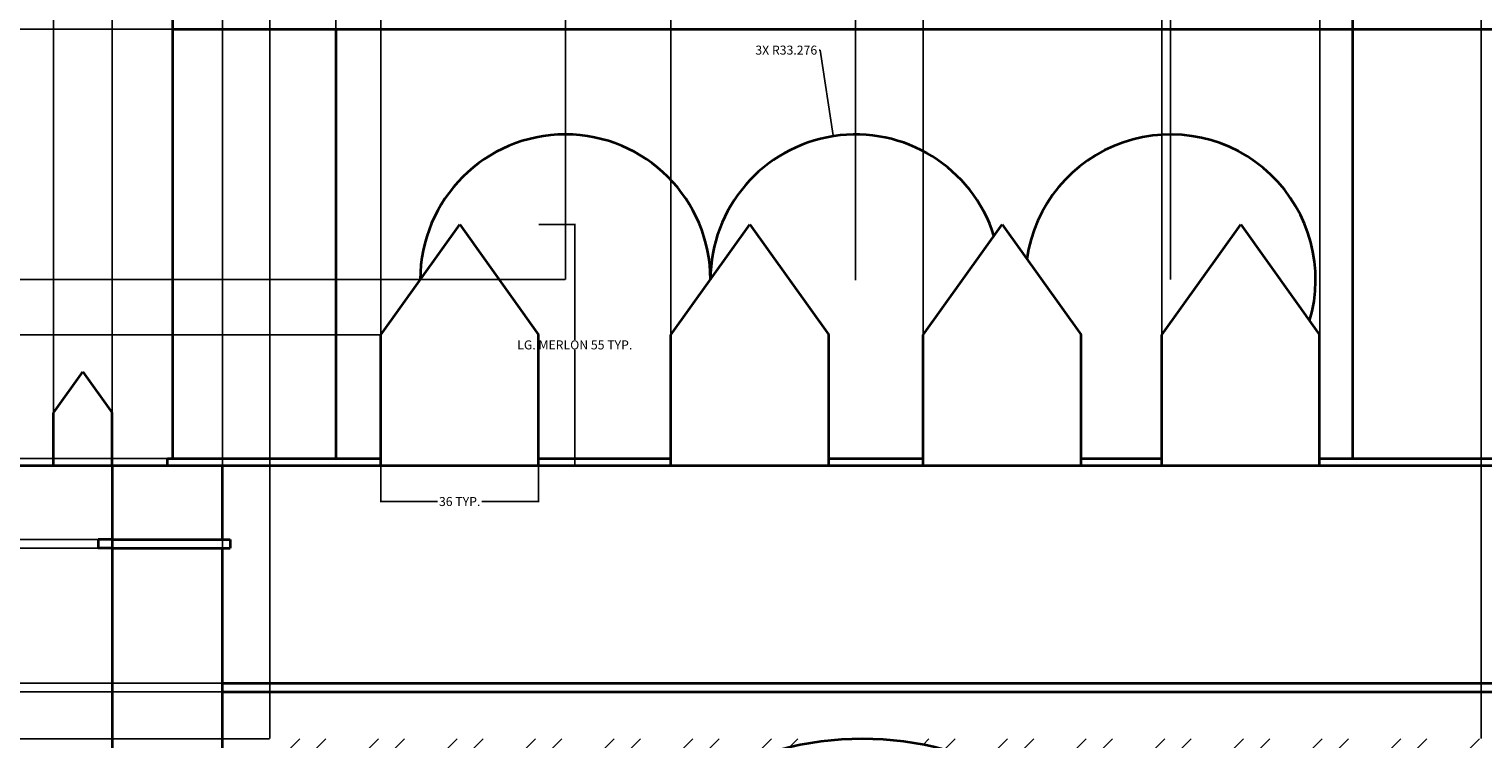
# Model space of a CAD drawing. Units: inches. Extents: x 14 to 859, y 52 to 711.
# Tile 5 of 11: x 244 to 577, y 342 to 504. Entities that reach past the tile are written whole.
import ezdxf

# ---------------------------------------------------------------- set-up
doc = ezdxf.new("R2010")
doc.units = ezdxf.units.IN
doc.header["$MEASUREMENT"] = 0
for name, color, linetype, lineweight in [('A-ANNO-DIMS', 2, 'Continuous', 18), ('A-ELEV', 7, 'Continuous', 35), ('A-ELEV-PATT', 8, 'Continuous', 13)]:
    doc.layers.add(name, color=color, linetype=linetype, lineweight=lineweight)
doc.styles.get("Standard").update_dxf_attribs({"font": 'arial.ttf'})
doc.dimstyles.get("Standard").update_dxf_attribs({"dimtxt": 2.0625, "dimasz": 0.18, "dimexe": 0.18, "dimexo": 0.0625, "dimgap": 0.09, "dimtad": 0, "dimtih": 1, "dimtoh": 1, "dimdec": 4, "dimzin": 0, "dimdsep": 46, "dimlunit": 4, "dimtxsty": 'Standard', "dimcen": 0.09, "dimadec": 0, "dimazin": 0, "dimtfac": 1, "dimtdec": 4, "dimtofl": 0, "dimtmove": 0, "dimatfit": 3, "dimfxl": 1, "dimtolj": 1, "dimtzin": 0, "dimarcsym": 0})

# ---------------------------------------------------------------- blocks, each defined once
blk = doc.blocks.new('MERLON-LARGE')
for p, q in [((0, 29.92), (18.11, 55.24)), ((18.11, 55.24), (36.21, 29.92)), ((0, 0), (0, 29.92)), ((36.21, 0), (36.21, 29.92))]:
    blk.add_line(p, q)
blk = doc.blocks.new('*D9')
at = {"layer": 'A-ANNO-DIMS', "color": 0, "lineweight": -2, "transparency": 16777216}
for p, q in [((360.45, 459.61), (368.85, 459.61)), ((368.67, 459.43), (368.67, 433.15)), ((368.67, 404.55), (368.67, 430.83)), ((360.45, 404.37), (368.85, 404.37))]:
    blk.add_line(p, q, dxfattribs=at)
at = {"layer": 'A-ANNO-DIMS', "color": 0, "transparency": 16777216}
for points in [[(368.64, 459.43), (368.7, 459.43), (368.67, 459.61)], [(368.64, 404.55), (368.7, 404.55), (368.67, 404.37)]]:
    blk.add_solid(points, dxfattribs=at)
at = {"layer": 'Defpoints', "color": 0, "transparency": 16777216}
for p in [(360.39, 459.61), (368.67, 459.61), (360.39, 404.37)]:
    blk.add_point(p, dxfattribs=at)
at = {"layer": 'A-ANNO-DIMS', "color": 0, "transparency": 16777216, "insert": (368.67, 431.99), "char_height": 2.0625, "attachment_point": 5}
blk.add_mtext('\\A1;LG. MERLON 55 TYP.', dxfattribs=at)
blk = doc.blocks.new('*D10')
at = {"layer": 'A-ANNO-DIMS', "color": 0, "lineweight": -2, "transparency": 16777216}
for p, q in [((324.18, 404.31), (324.18, 395.91)), ((360.39, 404.31), (360.39, 395.91)), ((324.36, 396.09), (337.17, 396.09)), ((360.21, 396.09), (347.39, 396.09))]:
    blk.add_line(p, q, dxfattribs=at)
at = {"layer": 'A-ANNO-DIMS', "color": 0, "transparency": 16777216}
for points in [[(324.36, 396.12), (324.36, 396.06), (324.18, 396.09)], [(360.21, 396.12), (360.21, 396.06), (360.39, 396.09)]]:
    blk.add_solid(points, dxfattribs=at)
at = {"layer": 'Defpoints', "color": 0, "transparency": 16777216}
for p in [(324.18, 404.37), (360.39, 404.37), (360.39, 396.09)]:
    blk.add_point(p, dxfattribs=at)
at = {"layer": 'A-ANNO-DIMS', "color": 0, "transparency": 16777216, "insert": (342.28, 396.09), "char_height": 2.0625, "attachment_point": 5}
blk.add_mtext('\\A1;36 TYP.', dxfattribs=at)
blk = doc.blocks.new('*D13')
at = {"layer": 'A-ANNO-DIMS', "color": 0, "lineweight": -2, "transparency": 16777216}
for p, q in [((60.78, 339.73), (60.78, 709.71)), ((60.96, 709.53), (432.6, 709.53)), ((811.37, 709.53), (439.73, 709.53)), ((811.55, 339.73), (811.55, 709.71))]:
    blk.add_line(p, q, dxfattribs=at)
at = {"layer": 'A-ANNO-DIMS', "color": 0, "transparency": 16777216}
for points in [[(60.96, 709.56), (60.96, 709.5), (60.78, 709.53)], [(811.37, 709.56), (811.37, 709.5), (811.55, 709.53)]]:
    blk.add_solid(points, dxfattribs=at)
at = {"layer": 'Defpoints', "color": 0, "transparency": 16777216}
for p in [(811.55, 709.53), (60.78, 339.66), (811.55, 339.66)]:
    blk.add_point(p, dxfattribs=at)
at = {"layer": 'A-ANNO-DIMS', "color": 0, "transparency": 16777216, "insert": (436.17, 709.53), "char_height": 2.062, "attachment_point": 5}
blk.add_mtext('\\A1;750.8', dxfattribs=at)
blk = doc.blocks.new('*D16')
at = {"layer": 'A-ANNO-DIMS', "color": 0, "lineweight": -2, "transparency": 16777216}
for p, q in [((429.96, 670.76), (17.7, 670.76)), ((17.88, 670.58), (17.88, 384.41)), ((17.88, 95.97), (17.88, 382.14)), ((60.72, 95.79), (17.7, 95.79))]:
    blk.add_line(p, q, dxfattribs=at)
at = {"layer": 'A-ANNO-DIMS', "color": 0, "transparency": 16777216}
for points in [[(17.85, 670.58), (17.91, 670.58), (17.88, 670.76)], [(17.85, 95.97), (17.91, 95.97), (17.88, 95.79)]]:
    blk.add_solid(points, dxfattribs=at)
at = {"layer": 'Defpoints', "color": 0, "transparency": 16777216}
for p in [(17.88, 670.76), (430.02, 670.76), (60.78, 95.79)]:
    blk.add_point(p, dxfattribs=at)
at = {"layer": 'A-ANNO-DIMS', "color": 0, "transparency": 16777216, "insert": (17.88, 383.28), "char_height": 2.062, "attachment_point": 5}
blk.add_mtext('\\A1;575', dxfattribs=at)
blk = doc.blocks.new('*D19')
at = {"layer": 'A-ANNO-DIMS', "color": 0, "lineweight": -2, "transparency": 16777216}
for p, q in [((430.09, 670.76), (854.64, 670.76)), ((854.46, 670.58), (854.46, 538.71)), ((854.46, 404.55), (854.46, 536.42)), ((609.81, 404.37), (854.64, 404.37))]:
    blk.add_line(p, q, dxfattribs=at)
at = {"layer": 'A-ANNO-DIMS', "color": 0, "transparency": 16777216}
for points in [[(854.43, 670.58), (854.49, 670.58), (854.46, 670.76)], [(854.43, 404.55), (854.49, 404.55), (854.46, 404.37)]]:
    blk.add_solid(points, dxfattribs=at)
at = {"layer": 'Defpoints', "color": 0, "transparency": 16777216}
for p in [(430.02, 670.76), (854.46, 670.76), (609.75, 404.37)]:
    blk.add_point(p, dxfattribs=at)
at = {"layer": 'A-ANNO-DIMS', "color": 0, "transparency": 16777216, "insert": (854.46, 537.57), "char_height": 2.062, "attachment_point": 5}
blk.add_mtext('\\A1;266.4', dxfattribs=at)
blk = doc.blocks.new('*D21')
at = {"layer": 'A-ANNO-DIMS', "color": 0, "lineweight": -2, "transparency": 16777216}
for p, q in [((287.89, 352.49), (287.89, 709.71)), ((288.07, 709.53), (289.04, 709.53)), ((298.55, 709.53), (297.59, 709.53)), ((298.73, 341.73), (298.73, 709.71))]:
    blk.add_line(p, q, dxfattribs=at)
at = {"layer": 'A-ANNO-DIMS', "color": 0, "transparency": 16777216}
for points in [[(288.07, 709.56), (288.07, 709.5), (287.89, 709.53)], [(298.55, 709.56), (298.55, 709.5), (298.73, 709.53)]]:
    blk.add_solid(points, dxfattribs=at)
at = {"layer": 'Defpoints', "color": 0, "transparency": 16777216}
for p in [(298.73, 709.53), (287.89, 352.43), (298.73, 341.67)]:
    blk.add_point(p, dxfattribs=at)
at = {"layer": 'A-ANNO-DIMS', "color": 0, "transparency": 16777216, "insert": (293.31, 709.53), "char_height": 2.062, "attachment_point": 5}
blk.add_mtext('\\A1;10.837', dxfattribs=at)
blk = doc.blocks.new('*D22')
at = {"layer": 'A-ANNO-DIMS', "color": 0, "lineweight": -2, "transparency": 16777216}
for p, q in [((298.73, 341.73), (298.73, 709.71)), ((298.91, 709.53), (434.03, 709.53)), ((576.33, 709.53), (441.21, 709.53)), ((576.51, 341.73), (576.51, 709.71))]:
    blk.add_line(p, q, dxfattribs=at)
at = {"layer": 'A-ANNO-DIMS', "color": 0, "transparency": 16777216}
for points in [[(298.91, 709.56), (298.91, 709.5), (298.73, 709.53)], [(576.33, 709.56), (576.33, 709.5), (576.51, 709.53)]]:
    blk.add_solid(points, dxfattribs=at)
at = {"layer": 'Defpoints', "color": 0, "transparency": 16777216}
for p in [(576.51, 709.53), (298.73, 341.67), (576.51, 341.67)]:
    blk.add_point(p, dxfattribs=at)
at = {"layer": 'A-ANNO-DIMS', "color": 0, "transparency": 16777216, "insert": (437.62, 709.53), "char_height": 2.062, "attachment_point": 5}
blk.add_mtext('\\A1;277.8', dxfattribs=at)
blk = doc.blocks.new('*D23')
at = {"layer": 'A-ANNO-DIMS', "color": 0, "lineweight": -2, "transparency": 16777216}
for p, q in [((576.51, 341.73), (576.51, 709.71)), ((576.69, 709.53), (576.9, 709.53)), ((584.26, 709.53), (584.04, 709.53)), ((584.44, 352.49), (584.44, 709.71))]:
    blk.add_line(p, q, dxfattribs=at)
at = {"layer": 'A-ANNO-DIMS', "color": 0, "transparency": 16777216}
for points in [[(576.69, 709.56), (576.69, 709.5), (576.51, 709.53)], [(584.26, 709.56), (584.26, 709.5), (584.44, 709.53)]]:
    blk.add_solid(points, dxfattribs=at)
at = {"layer": 'Defpoints', "color": 0, "transparency": 16777216}
for p in [(584.44, 709.53), (584.44, 352.43), (576.51, 341.67)]:
    blk.add_point(p, dxfattribs=at)
at = {"layer": 'A-ANNO-DIMS', "color": 0, "transparency": 16777216, "insert": (580.47, 709.53), "char_height": 2.062, "attachment_point": 5}
blk.add_mtext('\\A1;7.935', dxfattribs=at)
blk = doc.blocks.new('*D25')
at = {"layer": 'A-ANNO-DIMS', "color": 0, "lineweight": -2, "transparency": 16777216}
for p, q in [((298.67, 341.67), (17.7, 341.67)), ((17.88, 341.49), (17.88, 305.98)), ((17.88, 268.19), (17.88, 303.7)), ((298.67, 268.01), (17.7, 268.01))]:
    blk.add_line(p, q, dxfattribs=at)
at = {"layer": 'A-ANNO-DIMS', "color": 0, "transparency": 16777216}
for points in [[(17.85, 341.49), (17.91, 341.49), (17.88, 341.67)], [(17.85, 268.19), (17.91, 268.19), (17.88, 268.01)]]:
    blk.add_solid(points, dxfattribs=at)
at = {"layer": 'Defpoints', "color": 0, "transparency": 16777216}
for p in [(17.88, 341.67), (298.73, 341.67), (298.73, 268.01)]:
    blk.add_point(p, dxfattribs=at)
at = {"layer": 'A-ANNO-DIMS', "color": 0, "transparency": 16777216, "insert": (17.88, 304.84), "char_height": 2.062, "attachment_point": 5}
blk.add_mtext('\\A1;73.66', dxfattribs=at)
blk = doc.blocks.new('*D26')
at = {"layer": 'A-ANNO-DIMS', "color": 0, "lineweight": -2, "transparency": 16777216}
for p, q in [((287.83, 352.43), (17.7, 352.43)), ((17.88, 352.25), (17.88, 348.19)), ((17.88, 341.85), (17.88, 345.91)), ((298.67, 341.67), (17.7, 341.67))]:
    blk.add_line(p, q, dxfattribs=at)
at = {"layer": 'A-ANNO-DIMS', "color": 0, "transparency": 16777216}
for points in [[(17.85, 352.25), (17.91, 352.25), (17.88, 352.43)], [(17.85, 341.85), (17.91, 341.85), (17.88, 341.67)]]:
    blk.add_solid(points, dxfattribs=at)
at = {"layer": 'Defpoints', "color": 0, "transparency": 16777216}
for p in [(17.88, 352.43), (287.89, 352.43), (298.73, 341.67)]:
    blk.add_point(p, dxfattribs=at)
at = {"layer": 'A-ANNO-DIMS', "color": 0, "transparency": 16777216, "insert": (17.88, 347.05), "char_height": 2.062, "attachment_point": 5}
blk.add_mtext('\\A1;10.758', dxfattribs=at)
blk = doc.blocks.new('*D27')
at = {"layer": 'A-ANNO-DIMS', "color": 0, "lineweight": -2, "transparency": 16777216}
for p, q in [((287.83, 354.43), (17.7, 354.43)), ((17.88, 354.43), (17.88, 354.61)), ((17.88, 354.61), (18.06, 354.61)), ((17.88, 352.61), (17.88, 354.25)), ((287.83, 352.43), (17.7, 352.43))]:
    blk.add_line(p, q, dxfattribs=at)
at = {"layer": 'A-ANNO-DIMS', "color": 0, "transparency": 16777216}
for points in [[(17.85, 354.25), (17.91, 354.25), (17.88, 354.43)], [(17.85, 352.61), (17.91, 352.61), (17.88, 352.43)]]:
    blk.add_solid(points, dxfattribs=at)
at = {"layer": 'Defpoints', "color": 0, "transparency": 16777216}
for p in [(17.88, 354.43), (287.89, 354.43), (287.89, 352.43)]:
    blk.add_point(p, dxfattribs=at)
at = {"layer": 'A-ANNO-DIMS', "color": 0, "transparency": 16777216, "insert": (18.83, 354.61), "char_height": 2.062, "attachment_point": 5}
blk.add_mtext('\\A1;2', dxfattribs=at)
blk = doc.blocks.new('*D28')
at = {"layer": 'A-ANNO-DIMS', "color": 0, "lineweight": -2, "transparency": 16777216}
for p, q in [((289.61, 385.4), (17.7, 385.4)), ((17.88, 385.22), (17.88, 371.06)), ((17.88, 354.61), (17.88, 368.77)), ((287.83, 354.43), (17.7, 354.43))]:
    blk.add_line(p, q, dxfattribs=at)
at = {"layer": 'A-ANNO-DIMS', "color": 0, "transparency": 16777216}
for points in [[(17.85, 385.22), (17.91, 385.22), (17.88, 385.4)], [(17.85, 354.61), (17.91, 354.61), (17.88, 354.43)]]:
    blk.add_solid(points, dxfattribs=at)
at = {"layer": 'Defpoints', "color": 0, "transparency": 16777216}
for p in [(17.88, 385.4), (289.67, 385.4), (287.89, 354.43)]:
    blk.add_point(p, dxfattribs=at)
at = {"layer": 'A-ANNO-DIMS', "color": 0, "transparency": 16777216, "insert": (17.88, 369.91), "char_height": 2.062, "attachment_point": 5}
blk.add_mtext('\\A1;30.97', dxfattribs=at)
blk = doc.blocks.new('*D29')
at = {"layer": 'A-ANNO-DIMS', "color": 0, "lineweight": -2, "transparency": 16777216}
for p, q in [((289.61, 387.4), (17.7, 387.4)), ((17.88, 387.4), (17.88, 387.58)), ((17.88, 387.58), (18.06, 387.58)), ((17.88, 385.58), (17.88, 387.22)), ((289.61, 385.4), (17.7, 385.4))]:
    blk.add_line(p, q, dxfattribs=at)
at = {"layer": 'A-ANNO-DIMS', "color": 0, "transparency": 16777216}
for points in [[(17.85, 387.22), (17.91, 387.22), (17.88, 387.4)], [(17.85, 385.58), (17.91, 385.58), (17.88, 385.4)]]:
    blk.add_solid(points, dxfattribs=at)
at = {"layer": 'Defpoints', "color": 0, "transparency": 16777216}
for p in [(17.88, 387.4), (289.67, 387.4), (289.67, 385.4)]:
    blk.add_point(p, dxfattribs=at)
at = {"layer": 'A-ANNO-DIMS', "color": 0, "transparency": 16777216, "insert": (18.83, 387.58), "char_height": 2.062, "attachment_point": 5}
blk.add_mtext('\\A1;2', dxfattribs=at)
blk = doc.blocks.new('*D30')
at = {"layer": 'A-ANNO-DIMS', "color": 0, "lineweight": -2, "transparency": 16777216}
for p, q in [((287.83, 404.37), (17.7, 404.37)), ((17.88, 404.19), (17.88, 397.03)), ((17.88, 387.58), (17.88, 394.74)), ((289.61, 387.4), (17.7, 387.4))]:
    blk.add_line(p, q, dxfattribs=at)
at = {"layer": 'A-ANNO-DIMS', "color": 0, "transparency": 16777216}
for points in [[(17.85, 404.19), (17.91, 404.19), (17.88, 404.37)], [(17.85, 387.58), (17.91, 387.58), (17.88, 387.4)]]:
    blk.add_solid(points, dxfattribs=at)
at = {"layer": 'Defpoints', "color": 0, "transparency": 16777216}
for p in [(17.88, 404.37), (287.89, 404.37), (289.67, 387.4)]:
    blk.add_point(p, dxfattribs=at)
at = {"layer": 'A-ANNO-DIMS', "color": 0, "transparency": 16777216, "insert": (17.88, 395.88), "char_height": 2.062, "attachment_point": 5}
blk.add_mtext('\\A1;16.973', dxfattribs=at)
blk = doc.blocks.new('*D66')
at = {"layer": 'A-ANNO-DIMS', "color": 0, "lineweight": -2, "transparency": 16777216}
for p, q in [((223.53, 404.43), (223.53, 709.71)), ((223.71, 709.53), (232.77, 709.53)), ((249.01, 709.53), (239.95, 709.53)), ((249.19, 404.43), (249.19, 709.71))]:
    blk.add_line(p, q, dxfattribs=at)
at = {"layer": 'A-ANNO-DIMS', "color": 0, "transparency": 16777216}
for points in [[(223.71, 709.56), (223.71, 709.5), (223.53, 709.53)], [(249.01, 709.56), (249.01, 709.5), (249.19, 709.53)]]:
    blk.add_solid(points, dxfattribs=at)
at = {"layer": 'Defpoints', "color": 0, "transparency": 16777216}
for p in [(249.19, 709.53), (223.53, 404.37), (249.19, 404.37)]:
    blk.add_point(p, dxfattribs=at)
at = {"layer": 'A-ANNO-DIMS', "color": 0, "transparency": 16777216, "insert": (236.36, 709.53), "char_height": 2.062, "attachment_point": 5}
blk.add_mtext('\\A1;25.67', dxfattribs=at)
blk = doc.blocks.new('*D67')
at = {"layer": 'A-ANNO-DIMS', "color": 0, "lineweight": -2, "transparency": 16777216}
for p, q in [((249.19, 404.43), (249.19, 709.71)), ((249.37, 709.53), (252.41, 709.53)), ((262.4, 709.53), (259.36, 709.53)), ((262.58, 404.43), (262.58, 709.71))]:
    blk.add_line(p, q, dxfattribs=at)
at = {"layer": 'A-ANNO-DIMS', "color": 0, "transparency": 16777216}
for points in [[(249.37, 709.56), (249.37, 709.5), (249.19, 709.53)], [(262.4, 709.56), (262.4, 709.5), (262.58, 709.53)]]:
    blk.add_solid(points, dxfattribs=at)
at = {"layer": 'Defpoints', "color": 0, "transparency": 16777216}
for p in [(262.58, 709.53), (249.19, 404.37), (262.58, 404.37)]:
    blk.add_point(p, dxfattribs=at)
at = {"layer": 'A-ANNO-DIMS', "color": 0, "transparency": 16777216, "insert": (255.89, 709.53), "char_height": 2.062, "attachment_point": 5}
blk.add_mtext('\\A1;13.39', dxfattribs=at)
blk = doc.blocks.new('*D86')
at = {"layer": 'A-ANNO-DIMS', "color": 0, "lineweight": -2, "transparency": 16777216}
for p, q in [((366.44, 446.95), (17.7, 446.95)), ((17.88, 446.77), (17.88, 427.59)), ((17.88, 406.12), (17.88, 425.3)), ((276.44, 405.94), (17.7, 405.94))]:
    blk.add_line(p, q, dxfattribs=at)
at = {"layer": 'A-ANNO-DIMS', "color": 0, "transparency": 16777216}
for points in [[(17.85, 446.77), (17.91, 446.77), (17.88, 446.95)], [(17.85, 406.12), (17.91, 406.12), (17.88, 405.94)]]:
    blk.add_solid(points, dxfattribs=at)
at = {"layer": 'Defpoints', "color": 0, "transparency": 16777216}
for p in [(17.88, 446.95), (366.51, 446.95), (276.5, 405.94)]:
    blk.add_point(p, dxfattribs=at)
at = {"layer": 'A-ANNO-DIMS', "color": 0, "transparency": 16777216, "insert": (17.88, 426.45), "char_height": 2.062, "attachment_point": 5}
blk.add_mtext('\\A1;41.01', dxfattribs=at)
blk = doc.blocks.new('*D87')
at = {"layer": 'A-ANNO-DIMS', "color": 0, "lineweight": -2, "transparency": 16777216}
for p, q in [((276.44, 504.38), (17.7, 504.38)), ((17.88, 504.2), (17.88, 476.81)), ((17.88, 447.13), (17.88, 474.52)), ((366.44, 446.95), (17.7, 446.95))]:
    blk.add_line(p, q, dxfattribs=at)
at = {"layer": 'A-ANNO-DIMS', "color": 0, "transparency": 16777216}
for points in [[(17.85, 504.2), (17.91, 504.2), (17.88, 504.38)], [(17.85, 447.13), (17.91, 447.13), (17.88, 446.95)]]:
    blk.add_solid(points, dxfattribs=at)
at = {"layer": 'Defpoints', "color": 0, "transparency": 16777216}
for p in [(17.88, 504.38), (276.5, 504.38), (366.51, 446.95)]:
    blk.add_point(p, dxfattribs=at)
at = {"layer": 'A-ANNO-DIMS', "color": 0, "transparency": 16777216, "insert": (17.88, 475.67), "char_height": 2.062, "attachment_point": 5}
blk.add_mtext('\\A1;57.43', dxfattribs=at)
blk = doc.blocks.new('*D96')
at = {"layer": 'A-ANNO-DIMS', "color": 0, "lineweight": -2, "transparency": 16777216}
for p, q in [((313.86, 504.44), (313.86, 709.71)), ((314.04, 709.53), (336.61, 709.53)), ((366.33, 709.53), (343.76, 709.53)), ((366.51, 447.01), (366.51, 709.71))]:
    blk.add_line(p, q, dxfattribs=at)
at = {"layer": 'A-ANNO-DIMS', "color": 0, "transparency": 16777216}
for points in [[(314.04, 709.56), (314.04, 709.5), (313.86, 709.53)], [(366.33, 709.56), (366.33, 709.5), (366.51, 709.53)]]:
    blk.add_solid(points, dxfattribs=at)
at = {"layer": 'Defpoints', "color": 0, "transparency": 16777216}
for p in [(366.51, 709.53), (313.86, 504.38), (366.51, 446.95)]:
    blk.add_point(p, dxfattribs=at)
at = {"layer": 'A-ANNO-DIMS', "color": 0, "transparency": 16777216, "insert": (340.18, 709.53), "char_height": 2.062, "attachment_point": 5}
blk.add_mtext('\\A1;52.65', dxfattribs=at)
blk = doc.blocks.new('*D97')
at = {"layer": 'A-ANNO-DIMS', "color": 0, "lineweight": -2, "transparency": 16777216}
for p, q in [((366.51, 447.01), (366.51, 709.71)), ((366.69, 709.53), (396.2, 709.53)), ((432.88, 709.53), (403.37, 709.53)), ((433.06, 447.01), (433.06, 709.71))]:
    blk.add_line(p, q, dxfattribs=at)
at = {"layer": 'A-ANNO-DIMS', "color": 0, "transparency": 16777216}
for points in [[(366.69, 709.56), (366.69, 709.5), (366.51, 709.53)], [(432.88, 709.56), (432.88, 709.5), (433.06, 709.53)]]:
    blk.add_solid(points, dxfattribs=at)
at = {"layer": 'Defpoints', "color": 0, "transparency": 16777216}
for p in [(433.06, 709.53), (366.51, 446.95), (433.06, 446.95)]:
    blk.add_point(p, dxfattribs=at)
at = {"layer": 'A-ANNO-DIMS', "color": 0, "transparency": 16777216, "insert": (399.78, 709.53), "char_height": 2.062, "attachment_point": 5}
blk.add_mtext('\\A1;66.55', dxfattribs=at)
blk = doc.blocks.new('*D98')
at = {"layer": 'A-ANNO-DIMS', "color": 0, "lineweight": -2, "transparency": 16777216}
for p, q in [((433.06, 447.01), (433.06, 709.71)), ((433.24, 709.53), (465.59, 709.53)), ((505.07, 709.53), (472.72, 709.53)), ((505.25, 447.01), (505.25, 709.71))]:
    blk.add_line(p, q, dxfattribs=at)
at = {"layer": 'A-ANNO-DIMS', "color": 0, "transparency": 16777216}
for points in [[(433.24, 709.56), (433.24, 709.5), (433.06, 709.53)], [(505.07, 709.56), (505.07, 709.5), (505.25, 709.53)]]:
    blk.add_solid(points, dxfattribs=at)
at = {"layer": 'Defpoints', "color": 0, "transparency": 16777216}
for p in [(505.25, 709.53), (433.06, 446.95), (505.25, 446.95)]:
    blk.add_point(p, dxfattribs=at)
at = {"layer": 'A-ANNO-DIMS', "color": 0, "transparency": 16777216, "insert": (469.15, 709.53), "char_height": 2.062, "attachment_point": 5}
blk.add_mtext('\\A1;72.19', dxfattribs=at)
blk = doc.blocks.new('*D99')
at = {"layer": 'A-ANNO-DIMS', "color": 0, "lineweight": -2, "transparency": 16777216}
for p, q in [((505.25, 447.01), (505.25, 709.71)), ((505.43, 709.53), (521.76, 709.53)), ((546.91, 709.53), (530.58, 709.53)), ((547.09, 509.85), (547.09, 709.71))]:
    blk.add_line(p, q, dxfattribs=at)
at = {"layer": 'A-ANNO-DIMS', "color": 0, "transparency": 16777216}
for points in [[(505.43, 709.56), (505.43, 709.5), (505.25, 709.53)], [(546.91, 709.56), (546.91, 709.5), (547.09, 709.53)]]:
    blk.add_solid(points, dxfattribs=at)
at = {"layer": 'Defpoints', "color": 0, "transparency": 16777216}
for p in [(547.09, 709.53), (547.09, 509.79), (505.25, 446.95)]:
    blk.add_point(p, dxfattribs=at)
at = {"layer": 'A-ANNO-DIMS', "color": 0, "transparency": 16777216, "insert": (526.17, 709.53), "char_height": 2.062, "attachment_point": 5}
blk.add_mtext('\\A1;41.836', dxfattribs=at)
blk = doc.blocks.new('*D119')
at = {"layer": 'A-ANNO-DIMS', "color": 0, "lineweight": -2, "transparency": 16777216}
for p, q in [((287.89, 404.43), (287.89, 709.71)), ((288.07, 709.53), (301.66, 709.53)), ((324, 709.53), (310.41, 709.53)), ((324.18, 404.43), (324.18, 709.71))]:
    blk.add_line(p, q, dxfattribs=at)
at = {"layer": 'A-ANNO-DIMS', "color": 0, "transparency": 16777216}
for points in [[(288.07, 709.56), (288.07, 709.5), (287.89, 709.53)], [(324, 709.56), (324, 709.5), (324.18, 709.53)]]:
    blk.add_solid(points, dxfattribs=at)
at = {"layer": 'Defpoints', "color": 0, "transparency": 16777216}
for p in [(324.18, 709.53), (287.89, 404.37), (324.18, 404.37)]:
    blk.add_point(p, dxfattribs=at)
at = {"layer": 'A-ANNO-DIMS', "color": 0, "transparency": 16777216, "insert": (306.04, 709.53), "char_height": 2.062, "attachment_point": 5}
blk.add_mtext('\\A1;36.285', dxfattribs=at)
blk = doc.blocks.new('*D120')
at = {"layer": 'A-ANNO-DIMS', "color": 0, "lineweight": -2, "transparency": 16777216}
for p, q in [((324.18, 404.43), (324.18, 709.71)), ((324.36, 709.53), (353.87, 709.53)), ((390.55, 709.53), (361.04, 709.53)), ((390.73, 404.43), (390.73, 709.71))]:
    blk.add_line(p, q, dxfattribs=at)
at = {"layer": 'A-ANNO-DIMS', "color": 0, "transparency": 16777216}
for points in [[(324.36, 709.56), (324.36, 709.5), (324.18, 709.53)], [(390.55, 709.56), (390.55, 709.5), (390.73, 709.53)]]:
    blk.add_solid(points, dxfattribs=at)
at = {"layer": 'Defpoints', "color": 0, "transparency": 16777216}
for p in [(390.73, 709.53), (324.18, 404.37), (390.73, 404.37)]:
    blk.add_point(p, dxfattribs=at)
at = {"layer": 'A-ANNO-DIMS', "color": 0, "transparency": 16777216, "insert": (357.45, 709.53), "char_height": 2.062, "attachment_point": 5}
blk.add_mtext('\\A1;66.55', dxfattribs=at)
blk = doc.blocks.new('*D121')
at = {"layer": 'A-ANNO-DIMS', "color": 0, "lineweight": -2, "transparency": 16777216}
for p, q in [((390.73, 404.43), (390.73, 709.71)), ((390.91, 709.53), (416.86, 709.53)), ((448.36, 709.53), (422.4, 709.53)), ((448.54, 404.43), (448.54, 709.71))]:
    blk.add_line(p, q, dxfattribs=at)
at = {"layer": 'A-ANNO-DIMS', "color": 0, "transparency": 16777216}
for points in [[(390.91, 709.56), (390.91, 709.5), (390.73, 709.53)], [(448.36, 709.56), (448.36, 709.5), (448.54, 709.53)]]:
    blk.add_solid(points, dxfattribs=at)
at = {"layer": 'Defpoints', "color": 0, "transparency": 16777216}
for p in [(448.54, 709.53), (390.73, 404.37), (448.54, 404.37)]:
    blk.add_point(p, dxfattribs=at)
at = {"layer": 'A-ANNO-DIMS', "color": 0, "transparency": 16777216, "insert": (419.63, 709.53), "char_height": 2.062, "attachment_point": 5}
blk.add_mtext('\\A1;57.8', dxfattribs=at)
blk = doc.blocks.new('*D122')
at = {"layer": 'A-ANNO-DIMS', "color": 0, "lineweight": -2, "transparency": 16777216}
for p, q in [((448.54, 404.43), (448.54, 709.71)), ((448.72, 709.53), (473.12, 709.53)), ((503.05, 709.53), (478.65, 709.53)), ((503.23, 404.43), (503.23, 709.71))]:
    blk.add_line(p, q, dxfattribs=at)
at = {"layer": 'A-ANNO-DIMS', "color": 0, "transparency": 16777216}
for points in [[(448.72, 709.56), (448.72, 709.5), (448.54, 709.53)], [(503.05, 709.56), (503.05, 709.5), (503.23, 709.53)]]:
    blk.add_solid(points, dxfattribs=at)
at = {"layer": 'Defpoints', "color": 0, "transparency": 16777216}
for p in [(503.23, 709.53), (448.54, 404.37), (503.23, 404.37)]:
    blk.add_point(p, dxfattribs=at)
at = {"layer": 'A-ANNO-DIMS', "color": 0, "transparency": 16777216, "insert": (475.89, 709.53), "char_height": 2.062, "attachment_point": 5}
blk.add_mtext('\\A1;54.7', dxfattribs=at)
blk = doc.blocks.new('*D123')
at = {"layer": 'A-ANNO-DIMS', "color": 0, "lineweight": -2, "transparency": 16777216}
for p, q in [((539.45, 404.43), (539.45, 709.71)), ((539.63, 709.53), (558.42, 709.53)), ((584.44, 709.53), (565.64, 709.53)), ((584.62, 404.43), (584.62, 709.71))]:
    blk.add_line(p, q, dxfattribs=at)
at = {"layer": 'A-ANNO-DIMS', "color": 0, "transparency": 16777216}
for points in [[(539.63, 709.56), (539.63, 709.5), (539.45, 709.53)], [(584.44, 709.56), (584.44, 709.5), (584.62, 709.53)]]:
    blk.add_solid(points, dxfattribs=at)
at = {"layer": 'Defpoints', "color": 0, "transparency": 16777216}
for p in [(584.62, 709.53), (539.45, 404.37), (584.62, 404.37)]:
    blk.add_point(p, dxfattribs=at)
at = {"layer": 'A-ANNO-DIMS', "color": 0, "transparency": 16777216, "insert": (562.03, 709.53), "char_height": 2.062, "attachment_point": 5}
blk.add_mtext('\\A1;45.17', dxfattribs=at)
blk = doc.blocks.new('*D124')
at = {"layer": 'A-ANNO-DIMS', "color": 0, "lineweight": -2, "transparency": 16777216}
for p, q in [((324.12, 434.29), (17.7, 434.29)), ((17.88, 434.11), (17.88, 420.48)), ((17.88, 404.55), (17.88, 418.19)), ((324.12, 404.37), (17.7, 404.37))]:
    blk.add_line(p, q, dxfattribs=at)
at = {"layer": 'A-ANNO-DIMS', "color": 0, "transparency": 16777216}
for points in [[(17.85, 434.11), (17.91, 434.11), (17.88, 434.29)], [(17.85, 404.55), (17.91, 404.55), (17.88, 404.37)]]:
    blk.add_solid(points, dxfattribs=at)
at = {"layer": 'Defpoints', "color": 0, "transparency": 16777216}
for p in [(17.88, 434.29), (324.18, 434.29), (324.18, 404.37)]:
    blk.add_point(p, dxfattribs=at)
at = {"layer": 'A-ANNO-DIMS', "color": 0, "transparency": 16777216, "insert": (17.88, 419.33), "char_height": 2.062, "attachment_point": 5}
blk.add_mtext('\\A1;29.92', dxfattribs=at)
blk = doc.blocks.new('*D131')
at = {"layer": 'A-ANNO-DIMS', "color": 0, "lineweight": -2, "transparency": 16777216}
for p, q in [((424.73, 499.56), (424.91, 499.56)), ((424.91, 499.56), (427.94, 480.01)), ((432.97, 446.95), (433.15, 446.95)), ((433.06, 446.86), (433.06, 447.04))]:
    blk.add_line(p, q, dxfattribs=at)
at = {"layer": 'A-ANNO-DIMS', "color": 0, "transparency": 16777216}
blk.add_solid([(427.97, 480.02), (427.91, 480.01), (427.96, 479.83)], dxfattribs=at)
at = {"layer": 'Defpoints', "color": 0, "transparency": 16777216}
for p in [(427.96, 479.83), (433.06, 446.95)]:
    blk.add_point(p, dxfattribs=at)
at = {"layer": 'A-ANNO-DIMS', "color": 0, "transparency": 16777216, "insert": (417.16, 499.56), "char_height": 2.0625, "attachment_point": 5}
blk.add_mtext('\\A1;3X R33.276', dxfattribs=at)

msp = doc.modelspace()

# ---------------------------------------------------------------- hatches: boundary and pattern name
at = {"layer": 'A-ELEV-PATT'}
h = msp.add_hatch(dxfattribs=at)
h.set_pattern_fill('ANSI32', color=256, scale=34)
h.paths.add_polyline_path([(434.5861, 341.6716, 0.41417057), (360.935, 268.0097), (295.7375, 268.0097), (295.7375, 265.9828), (298.7295, 265.9828), (362.2006, 265.9828), (365.3206, 265.8525), (362.2006, 265.8525), (298.7295, 265.9828), (295.7375, 265.9828), (295.7375, 268.0097), (298.7295, 268.0097), (298.7295, 341.6716)])
h.paths.add_polyline_path([(576.5058, 341.6716), (570.5754, 341.6716), (434.5861, 341.6716, -0.41433672), (508.2589, 267.9895), (576.5058, 267.9895)])

# ---------------------------------------------------------------- linework, layer by layer
at = {"layer": 'A-ELEV'}
for p, q in [((276.5038, 405.9412), (276.5038, 509.7903)), ((547.0851, 405.9412), (547.0851, 509.7903)), ((276.5038, 504.3815), (537.6873, 504.3815)), ((313.8595, 504.3815), (313.8595, 405.9412)), ((536.2033, 504.3815), (584.4409, 504.3815)), ((249.1939, 416.4248), (255.8888, 425.7853)), ((255.8888, 425.7853), (262.5837, 416.4248)), ((249.1939, 404.3712), (249.1939, 416.4248)), ((262.5837, 404.3712), (262.5837, 416.4248)), ((140.5683, 404.3712), (262.6537, 404.3712)), ((262.6537, 370.2389), (262.6537, 404.3712)), ((262.6537, 404.3712), (287.893, 404.3712)), ((275.2733, 404.3712), (275.2733, 405.9412)), ((275.2733, 405.9412), (307.522, 405.9412)), ((287.893, 387.3985), (287.893, 404.3712)), ((287.893, 404.3712), (376.0525, 404.3712)), ((307.522, 405.9412), (318.7414, 405.9412)), ((318.7414, 405.9412), (324.1777, 405.9412)), ((360.389, 405.9412), (373.4249, 405.9412)), ((373.4249, 405.9412), (390.7307, 405.9412)), ((376.0525, 404.3712), (584.619, 404.3712)), ((426.9419, 405.9412), (448.5359, 405.9412)), ((484.7472, 405.9412), (503.2347, 405.9412)), ((539.446, 405.9412), (584.4409, 405.9412)), ((262.6537, 387.3985), (259.4218, 387.3985)), ((259.4218, 387.3985), (259.4218, 385.3985)), ((262.6537, 387.3985), (287.893, 387.3985)), ((287.893, 387.3985), (289.67, 387.3985)), ((289.67, 387.3985), (289.67, 385.3985)), ((262.6537, 385.3985), (259.4218, 385.3985)), ((262.6537, 385.3985), (287.893, 385.3985)), ((287.893, 371.6812), (287.893, 385.3985)), ((287.893, 385.3985), (289.67, 385.3985)), ((262.6537, 339.6626), (262.6537, 370.2389)), ((287.893, 304.6217), (287.893, 371.6812)), ((287.893, 354.4291), (584.4409, 354.4291)), ((287.893, 352.4291), (584.4409, 352.4291))]:
    msp.add_line(p, q, dxfattribs=at)
for centre, radius, start, end in [((366.507, 446.9501), 33.2765, 0, 180), ((433.06, 446.9501), 33.2765, 17.588726, 180), ((505.2493, 446.9501), 33.2765, 343.495253, 171.8269), ((434.5969, 268.0097), 73.6619, 359.983178, 180)]:
    msp.add_arc(centre, radius, start, end, dxfattribs=at)

# ---------------------------------------------------------------- block references
for p in [(324.178, 404.371), (390.731, 404.371), (448.5362, 404.371), (503.235, 404.371)]:
    msp.add_blockref('MERLON-LARGE', p, dxfattribs=at)

# ---------------------------------------------------------------- dimensions: what is measured, and where the dimension line sits
at = {"layer": 'A-ANNO-DIMS'}
for base, p1, p2, override, picture, middle in [((811.5534, 709.5262), (60.7804, 339.6626), (811.5534, 339.6626), {"dimdec": 1, "dimlfac": 1, "dimrnd": 0, "dimzin": 0, "dimdsep": 46, "dimlunit": 2}, '*D13', (436.1669, 709.5262)), ((249.1939, 709.5262), (223.5256, 404.3712), (249.1939, 404.3712), {"dimdec": 2, "dimlfac": 1, "dimrnd": 0, "dimzin": 0, "dimdsep": 46, "dimlunit": 2}, '*D66', (236.3598, 709.5262)), ((262.5837, 709.5262), (249.1939, 404.3712), (262.5837, 404.3712), {"dimdec": 2, "dimlfac": 1, "dimrnd": 0, "dimzin": 0, "dimdsep": 46, "dimlunit": 2}, '*D67', (255.8888, 709.5262)), ((298.72949, 709.52622), (287.89298, 352.42914), (298.72949, 341.67161), {"dimdec": 3, "dimlfac": 1, "dimrnd": 0, "dimzin": 0, "dimdsep": 46, "dimlunit": 2}, '*D21', (293.31124, 709.52622)), ((324.1777, 709.5262), (287.893, 404.3712), (324.1777, 404.3712), {"dimdec": 3, "dimlfac": 1, "dimrnd": 0, "dimzin": 0, "dimdsep": 46, "dimlunit": 2}, '*D119', (306.0353, 709.5262)), ((576.5058, 709.5262), (298.7295, 341.6716), (576.5058, 341.6716), {"dimdec": 1, "dimlfac": 1, "dimrnd": 0, "dimzin": 0, "dimdsep": 46, "dimlunit": 2}, '*D22', (437.6176, 709.5262)), ((366.507, 709.5262), (313.8595, 504.3815), (366.507, 446.9501), {"dimdec": 2, "dimlfac": 1, "dimrnd": 0, "dimzin": 0, "dimdsep": 46, "dimlunit": 2}, '*D96', (340.1833, 709.5262)), ((390.7307, 709.5262), (324.1777, 404.3712), (390.7307, 404.3712), {"dimdec": 2, "dimlfac": 1, "dimrnd": 0, "dimzin": 0, "dimdsep": 46, "dimlunit": 2}, '*D120', (357.4542, 709.5262)), ((433.06, 709.5262), (366.507, 446.9501), (433.06, 446.9501), {"dimdec": 2, "dimlfac": 1, "dimrnd": 0, "dimzin": 0, "dimdsep": 46, "dimlunit": 2}, '*D97', (399.7835, 709.5262)), ((448.5359, 709.5262), (390.7307, 404.3712), (448.5359, 404.3712), {"dimdec": 1, "dimlfac": 1, "dimrnd": 0, "dimzin": 0, "dimdsep": 46, "dimlunit": 2}, '*D121', (419.6333, 709.5262)), ((505.2493, 709.5262), (433.06, 446.9501), (505.2493, 446.9501), {"dimdec": 2, "dimlfac": 1, "dimrnd": 0, "dimzin": 0, "dimdsep": 46, "dimlunit": 2}, '*D98', (469.1547, 709.5262)), ((503.2347, 709.5262), (448.5359, 404.3712), (503.2347, 404.3712), {"dimdec": 1, "dimlfac": 1, "dimrnd": 0, "dimzin": 0, "dimdsep": 46, "dimlunit": 2}, '*D122', (475.8853, 709.5262)), ((547.0851, 709.5262), (505.2493, 446.9501), (547.0851, 509.7903), {"dimdec": 3, "dimlfac": 1, "dimrnd": 0, "dimzin": 0, "dimdsep": 46, "dimlunit": 2}, '*D99', (526.1672, 709.5262)), ((584.619, 709.5262), (539.446, 404.3712), (584.619, 404.3712), {"dimdec": 2, "dimlfac": 1, "dimrnd": 0, "dimzin": 0, "dimdsep": 46, "dimlunit": 2}, '*D123', (562.0325, 709.5262)), ((584.4409, 709.5262), (576.5058, 341.6716), (584.4409, 352.4291), {"dimdec": 3, "dimlfac": 1, "dimrnd": 0, "dimzin": 0, "dimdsep": 46, "dimlunit": 2}, '*D23', (580.4733, 709.5262))]:
    dim = msp.add_linear_dim(base=base, p1=p1, p2=p2, dimstyle='Standard', override=override, dxfattribs=at)
    dim.commit()
    dim.dimension.update_dxf_attribs({"geometry": picture, "text_midpoint": middle})
for base, p1, p2, override, picture, middle in [((17.8785, 670.7637), (60.7804, 95.7876), (430.0228, 670.7637), {"dimdec": 0, "dimlfac": 1, "dimrnd": 0, "dimzin": 0, "dimdsep": 46, "dimlunit": 2}, '*D16', (17.8785, 383.2756)), ((854.4554, 670.7637), (609.7501, 404.3712), (430.0228, 670.7637), {"dimdec": 1, "dimlfac": 1, "dimrnd": 0, "dimzin": 0, "dimdsep": 46, "dimlunit": 2}, '*D19', (854.4554, 537.5675)), ((17.8785, 504.3815), (366.507, 446.9501), (276.5038, 504.3815), {"dimdec": 2, "dimlfac": 1, "dimrnd": 0, "dimzin": 0, "dimdsep": 46, "dimlunit": 2}, '*D87', (17.8785, 475.6658)), ((17.8785, 446.9501), (276.5038, 405.9412), (366.507, 446.9501), {"dimdec": 2, "dimlfac": 1, "dimrnd": 0, "dimzin": 0, "dimdsep": 46, "dimlunit": 2}, '*D86', (17.8785, 426.4456)), ((17.8785, 434.2929), (324.1777, 404.3712), (324.1777, 434.2929), {"dimdec": 2, "dimlfac": 1, "dimrnd": 0, "dimzin": 0, "dimdsep": 46, "dimlunit": 2}, '*D124', (17.8785, 419.332)), ((17.8785, 404.3712), (289.67, 387.3985), (287.893, 404.3712), {"dimdec": 3, "dimlfac": 1, "dimrnd": 0, "dimzin": 0, "dimdsep": 46, "dimlunit": 2}, '*D30', (17.8785, 395.8849)), ((17.8785, 387.3985), (289.67, 385.3985), (289.67, 387.3985), {"dimdec": 0, "dimlfac": 1, "dimrnd": 0, "dimzin": 0, "dimdsep": 46, "dimlunit": 2}, '*D29', (18.8315, 387.5785)), ((17.8785, 385.3985), (287.893, 354.4291), (289.67, 385.3985), {"dimdec": 2, "dimlfac": 1, "dimrnd": 0, "dimzin": 0, "dimdsep": 46, "dimlunit": 2}, '*D28', (17.8785, 369.9138)), ((17.8785, 354.4291), (287.893, 352.4291), (287.893, 354.4291), {"dimdec": 0, "dimlfac": 1, "dimrnd": 0, "dimzin": 0, "dimdsep": 46, "dimlunit": 2}, '*D27', (18.8315, 354.6091)), ((17.87849, 352.42914), (298.72949, 341.67161), (287.89298, 352.42914), {"dimdec": 3, "dimlfac": 1, "dimrnd": 0, "dimzin": 0, "dimdsep": 46, "dimlunit": 2}, '*D26', (17.87849, 347.05038)), ((17.8785, 341.6716), (298.7295, 268.0097), (298.7295, 341.6716), {"dimdec": 2, "dimlfac": 1, "dimrnd": 0, "dimzin": 0, "dimdsep": 46, "dimlunit": 2}, '*D25', (17.8785, 304.8406))]:
    dim = msp.add_linear_dim(base=base, p1=p1, p2=p2, angle=90, dimstyle='Standard', override=override, dxfattribs=at)
    dim.commit()
    dim.dimension.update_dxf_attribs({"geometry": picture, "text_midpoint": middle})
dim = msp.add_radius_dim(center=(433.06, 446.9501), mpoint=(427.9647, 479.8341), text='3X <>', dimstyle='Standard', override={"dimdec": 3, "dimlfac": 1, "dimrnd": 0, "dimzin": 0, "dimdsep": 46, "dimlunit": 2}, dxfattribs=at)
dim.commit()
dim.dimension.update_dxf_attribs({"geometry": '*D131', "text_midpoint": (417.155, 499.5646), "dimtype": 164})
dim = msp.add_linear_dim(base=(368.6744, 459.6073), p1=(360.389, 404.3712), p2=(360.389, 459.6073), angle=90, text='LG. MERLON <> TYP.', dimstyle='Standard', override={"dimdec": 0, "dimlfac": 1, "dimrnd": 0, "dimzin": 0, "dimdsep": 46, "dimlunit": 2}, dxfattribs=at)
dim.commit()
dim.dimension.update_dxf_attribs({"geometry": '*D9', "text_midpoint": (368.6744, 431.9893)})
dim = msp.add_linear_dim(base=(360.389, 396.0858), p1=(324.1777, 404.3712), p2=(360.389, 404.3712), text='<> TYP.', dimstyle='Standard', override={"dimdec": 0, "dimlfac": 1, "dimrnd": 0, "dimzin": 0, "dimdsep": 46, "dimlunit": 2}, dxfattribs=at)
dim.commit()
dim.dimension.update_dxf_attribs({"geometry": '*D10', "text_midpoint": (342.2833, 396.0858)})

doc.saveas('drawing.dxf')
